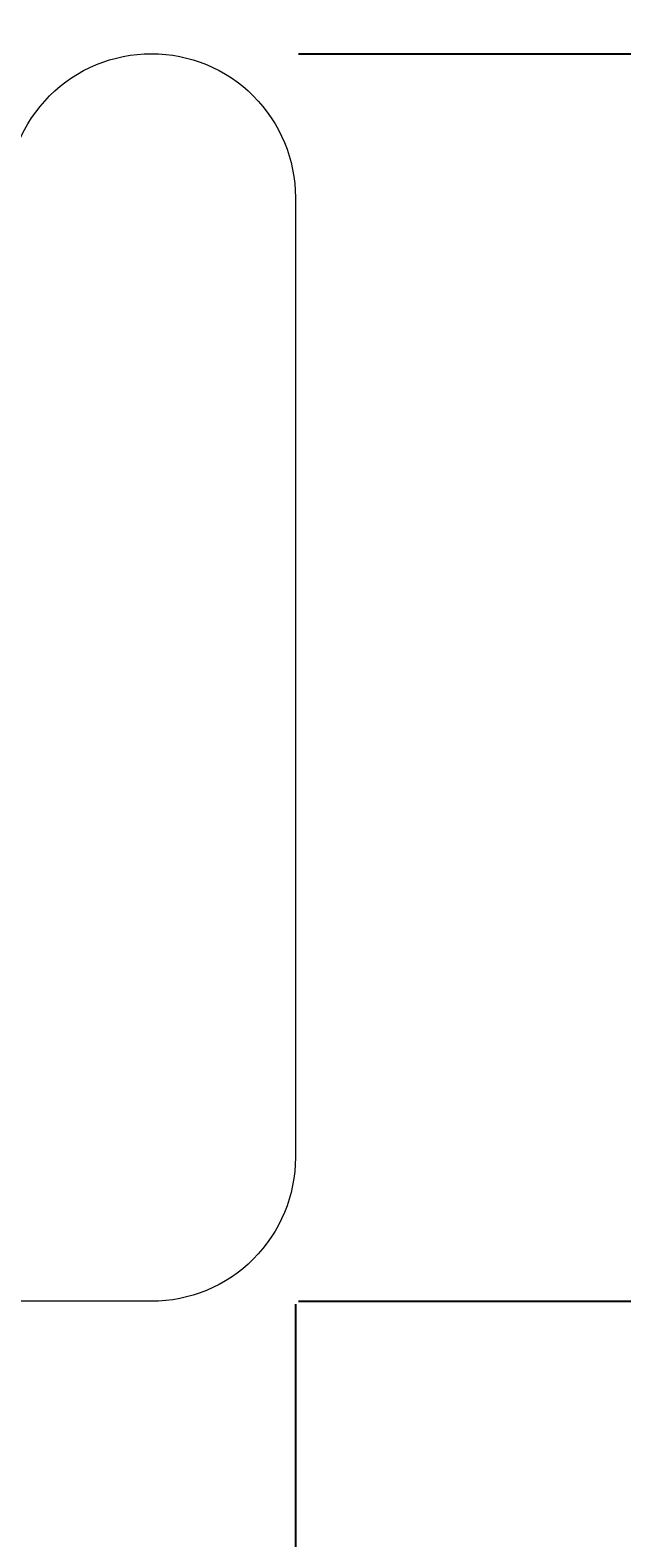
# Model space of a CAD drawing. Units: inches. Extents: x -61 to 1599, y -1316 to 257.
# Tile 108 of 204: x 224 to 236, y -166 to -135. Entities that reach past the tile are written whole.
import ezdxf

# ---------------------------------------------------------------- set-up
doc = ezdxf.new("R2010")
doc.units = ezdxf.units.IN
doc.header["$MEASUREMENT"] = 0
doc.layers.add('A-ANNO-DIMS', color=2, linetype='Continuous', lineweight=18)
doc.layers.add('FURNITURE', color=83, linetype='Continuous', lineweight=18)
doc.styles.get("Standard").update_dxf_attribs({"font": 'arial.ttf'})
doc.dimstyles.get("Standard").update_dxf_attribs({"dimtxt": 0.18, "dimasz": 0.18, "dimexe": 0.18, "dimexo": 0.0625, "dimgap": 0.09, "dimtad": 0, "dimtih": 1, "dimtoh": 1, "dimdec": 0, "dimzin": 0, "dimdsep": 46, "dimlunit": 3, "dimtxsty": 'Standard', "dimcen": 0.09, "dimadec": 0, "dimazin": 0, "dimtfac": 1, "dimtdec": 0, "dimtofl": 0, "dimtmove": 0, "dimatfit": 3, "dimfxl": 1, "dimtolj": 1, "dimtzin": 0, "dimarcsym": 0})

# ---------------------------------------------------------------- blocks, each defined once
blk = doc.blocks.new('SOFA-THREE-SEAT')
blk.add_lwpolyline([(78, 8.382), (78, 23, -0.414214), (81, 26), (81, 26, -0.414214), (84, 23), (84, 3, -0.414214), (81, 0), (3, 0, -0.414214), (0, 3), (0, 23, -0.414214), (3, 26), (3, 26, -0.414214), (6, 23), (6, 8.382, 0.414214), (9, 5.382), (75, 5.382, 0.414214)], format="xyb", close=True)
blk = doc.blocks.new('*D670')
at = {"layer": 'A-ANNO-DIMS', "color": 0, "lineweight": -2, "transparency": 16777216}
for p, q in [((145.375, -161.442), (145.375, -174.159)), ((229.375, -161.442), (229.375, -174.159)), ((145.555, -173.979), (186.47, -173.979)), ((229.195, -173.979), (188.279, -173.979))]:
    blk.add_line(p, q, dxfattribs=at)
at = {"layer": 'A-ANNO-DIMS', "color": 0, "transparency": 16777216}
for points in [[(145.555, -173.949), (145.555, -174.009), (145.375, -173.979)], [(229.195, -173.949), (229.195, -174.009), (229.375, -173.979)]]:
    blk.add_solid(points, dxfattribs=at)
at = {"layer": 'DEFPOINTS', "color": 0, "transparency": 16777216}
for p in [(145.375, -161.379), (229.375, -161.379), (229.375, -173.979)]:
    blk.add_point(p, dxfattribs=at)
at = {"layer": 'A-ANNO-DIMS', "color": 0, "transparency": 16777216, "insert": (187.375, -173.979), "char_height": 0.18, "attachment_point": 5}
blk.add_mtext('\\A1;SOFA 84 TYP.', dxfattribs=at)
blk = doc.blocks.new('*D671')
at = {"layer": 'A-ANNO-DIMS', "color": 0, "lineweight": -2, "transparency": 16777216}
for p, q in [((229.437, -135.379), (242.155, -135.379)), ((241.975, -135.559), (241.975, -148.197)), ((241.975, -161.199), (241.975, -148.561)), ((229.437, -161.379), (242.155, -161.379))]:
    blk.add_line(p, q, dxfattribs=at)
at = {"layer": 'A-ANNO-DIMS', "color": 0, "transparency": 16777216}
for points in [[(241.945, -135.559), (242.005, -135.559), (241.975, -135.379)], [(241.945, -161.199), (242.005, -161.199), (241.975, -161.379)]]:
    blk.add_solid(points, dxfattribs=at)
at = {"layer": 'DEFPOINTS', "color": 0, "transparency": 16777216}
for p in [(229.375, -135.379), (241.975, -135.379), (229.375, -161.379)]:
    blk.add_point(p, dxfattribs=at)
at = {"layer": 'A-ANNO-DIMS', "color": 0, "transparency": 16777216, "insert": (241.975, -148.379), "char_height": 0.18, "attachment_point": 5}
blk.add_mtext('\\A1;26 TYP.', dxfattribs=at)
blk = doc.blocks.new('*D687')
at = {"layer": 'A-ANNO-DIMS', "color": 0, "lineweight": -2, "transparency": 16777216}
for p, q in [((289.418, 181.677), (-61.077, 181.677)), ((-60.897, 181.497), (-60.897, -528.952)), ((-60.897, -1239.765), (-60.897, -529.316)), ((319.64, -1239.945), (-61.077, -1239.945))]:
    blk.add_line(p, q, dxfattribs=at)
at = {"layer": 'A-ANNO-DIMS', "color": 0, "transparency": 16777216}
for points in [[(-60.927, 181.497), (-60.867, 181.497), (-60.897, 181.677)], [(-60.927, -1239.765), (-60.867, -1239.765), (-60.897, -1239.945)]]:
    blk.add_solid(points, dxfattribs=at)
at = {"layer": 'DEFPOINTS', "color": 0, "transparency": 16777216}
for p in [(289.481, 181.677), (-60.897, -1239.945), (319.703, -1239.945)]:
    blk.add_point(p, dxfattribs=at)
at = {"layer": 'A-ANNO-DIMS', "color": 0, "transparency": 16777216, "insert": (-60.897, -529.134), "char_height": 0.18, "attachment_point": 5}
blk.add_mtext('\\A1;1421.6', dxfattribs=at)
blk = doc.blocks.new('*D701')
at = {"layer": 'A-ANNO-DIMS', "color": 0, "lineweight": -2, "transparency": 16777216}
for p, q in [((215.752, -616.882), (215.752, 257.457)), ((252.882, -616.882), (252.882, 257.457)), ((215.932, 257.277), (233.924, 257.277)), ((252.702, 257.277), (234.711, 257.277))]:
    blk.add_line(p, q, dxfattribs=at)
at = {"layer": 'A-ANNO-DIMS', "color": 0, "transparency": 16777216}
for points in [[(215.932, 257.307), (215.932, 257.247), (215.752, 257.277)], [(252.702, 257.307), (252.702, 257.247), (252.882, 257.277)]]:
    blk.add_solid(points, dxfattribs=at)
at = {"layer": 'DEFPOINTS', "color": 0, "transparency": 16777216}
for p in [(252.882, 257.277), (215.752, -616.945), (252.882, -616.945)]:
    blk.add_point(p, dxfattribs=at)
at = {"layer": 'A-ANNO-DIMS', "color": 0, "transparency": 16777216, "insert": (234.317, 257.277), "char_height": 0.18, "attachment_point": 5}
blk.add_mtext('\\A1;37.13', dxfattribs=at)

msp = doc.modelspace()

# ---------------------------------------------------------------- block references
at = {"layer": 'FURNITURE'}
msp.add_blockref('SOFA-THREE-SEAT', (145.375, -161.379), dxfattribs=at)

# ---------------------------------------------------------------- dimensions: what is measured, and where the dimension line sits
at = {"layer": 'A-ANNO-DIMS'}
dim = msp.add_linear_dim(base=(252.8825, 257.2771), p1=(215.7521, -616.9446), p2=(252.8825, -616.9446), dimstyle='Standard', override={"dimdec": 2, "dimlfac": 1, "dimrnd": 0, "dimzin": 0, "dimdsep": 46, "dimlunit": 2}, dxfattribs=at)
dim.commit()
dim.dimension.update_dxf_attribs({"geometry": '*D701', "text_midpoint": (234.3173, 257.2771)})
dim = msp.add_linear_dim(base=(-60.8972, -1239.9446), p1=(289.4807, 181.6771), p2=(319.7028, -1239.9446), angle=90, dimstyle='Standard', override={"dimdec": 1, "dimlfac": 1, "dimrnd": 0, "dimzin": 0, "dimdsep": 46, "dimlunit": 2}, dxfattribs=at)
dim.commit()
dim.dimension.update_dxf_attribs({"geometry": '*D687', "text_midpoint": (-60.8972, -529.1337)})
dim = msp.add_linear_dim(base=(241.9746, -135.3792), p1=(229.3746, -161.3792), p2=(229.3746, -135.3792), angle=90, text='<> TYP.', dimstyle='Standard', override={"dimdec": 0, "dimlfac": 1, "dimrnd": 0, "dimzin": 0, "dimdsep": 46, "dimlunit": 2}, dxfattribs=at)
dim.commit()
dim.dimension.update_dxf_attribs({"geometry": '*D671', "text_midpoint": (241.9746, -148.3792)})
dim = msp.add_linear_dim(base=(229.3746, -173.9792), p1=(145.3746, -161.3792), p2=(229.3746, -161.3792), text='SOFA <> TYP.', dimstyle='Standard', override={"dimdec": 0, "dimlfac": 1, "dimrnd": 0, "dimzin": 0, "dimdsep": 46, "dimlunit": 2}, dxfattribs=at)
dim.commit()
dim.dimension.update_dxf_attribs({"geometry": '*D670', "text_midpoint": (187.3746, -173.9792)})

doc.saveas('drawing.dxf')
